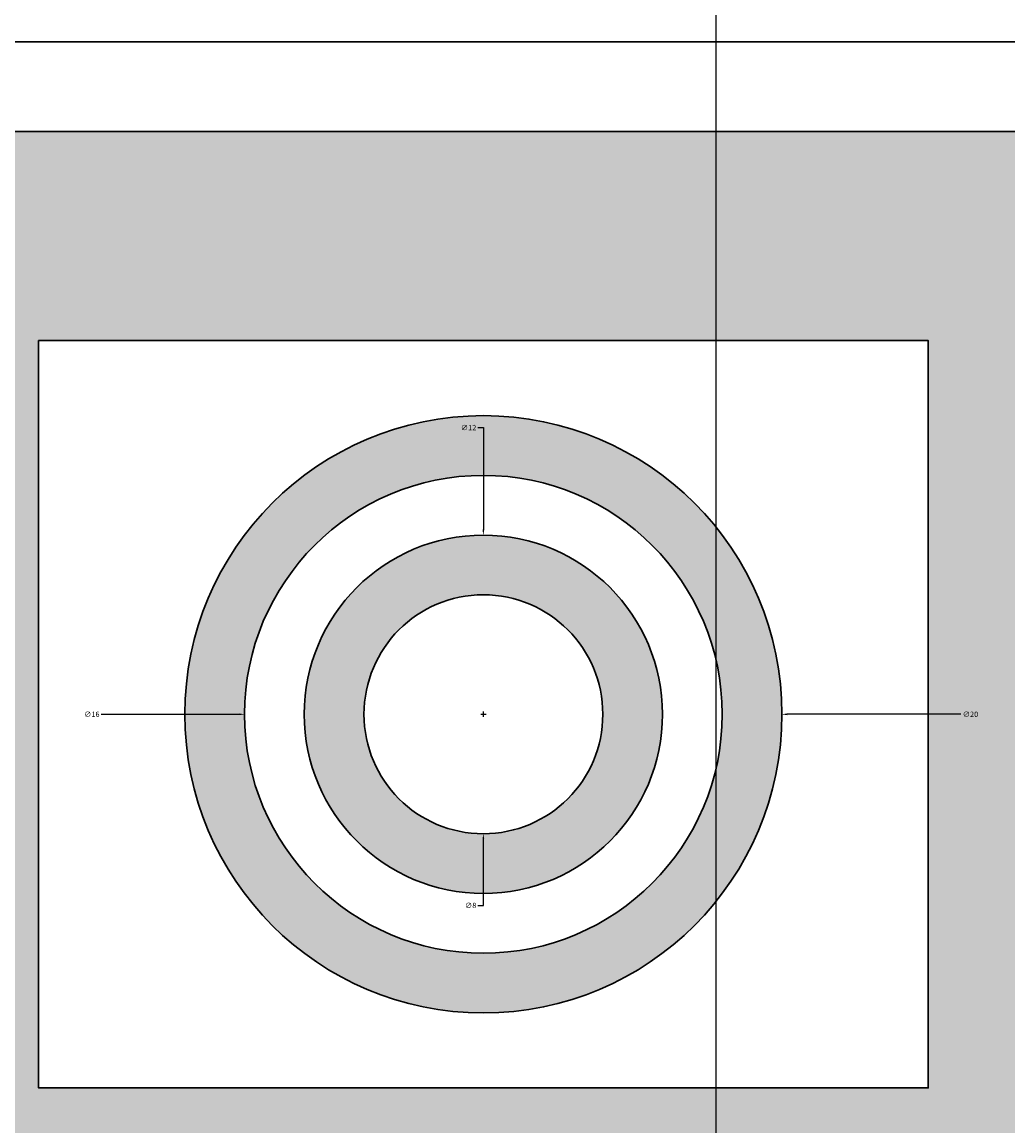
# Model space of a CAD drawing. Units: millimetres. Extents: x -8 to 285, y 5 to 221.
# Tile 20 of 30: x 208 to 241, y 66 to 103. Entities that reach past the tile are written whole.
import ezdxf

# ---------------------------------------------------------------- set-up
doc = ezdxf.new("R2010")
doc.units = ezdxf.units.MM
for name, color, linetype, lineweight in [('A-ANNO-DIMS', 2, 'Continuous', 18), ('E-EQPM-PATT', 252, 'Continuous', 13), ('E-POWR-INVR', 7, 'Continuous', 30)]:
    doc.layers.add(name, color=color, linetype=linetype, lineweight=lineweight)
doc.styles.get("Standard").update_dxf_attribs({"font": 'arial.ttf'})
doc.dimstyles.get("Standard").update_dxf_attribs({"dimtxt": 0.18, "dimasz": 0.18, "dimexe": 0.18, "dimexo": 0.0625, "dimgap": 0.09, "dimtad": 0, "dimtih": 1, "dimtoh": 1, "dimdec": 4, "dimzin": 0, "dimdsep": 46, "dimtxsty": 'Standard', "dimcen": 0.09, "dimadec": 0, "dimazin": 0, "dimtfac": 1, "dimtdec": 4, "dimtofl": 0, "dimtmove": 0, "dimatfit": 3, "dimfxl": 1, "dimtolj": 1, "dimtzin": 0, "dimarcsym": 0})

# ---------------------------------------------------------------- blocks, each defined once
blk = doc.blocks.new('*D14')
at = {"layer": 'A-ANNO-DIMS', "color": 0, "lineweight": -2, "transparency": 16777216}
for p, q in [((189.039, 137.013), (189.039, 5.222)), ((230.967, 137.013), (230.967, 5.222)), ((189.219, 5.402), (209.606, 5.402)), ((230.787, 5.402), (210.4, 5.402))]:
    blk.add_line(p, q, dxfattribs=at)
at = {"layer": 'A-ANNO-DIMS', "color": 0, "transparency": 16777216}
for points in [[(189.219, 5.432), (189.219, 5.372), (189.039, 5.402)], [(230.787, 5.432), (230.787, 5.372), (230.967, 5.402)]]:
    blk.add_solid(points, dxfattribs=at)
at = {"layer": 'Defpoints', "color": 0, "transparency": 16777216}
for p in [(189.039, 137.075), (230.967, 137.075), (230.967, 5.402)]:
    blk.add_point(p, dxfattribs=at)
at = {"layer": 'A-ANNO-DIMS', "color": 0, "transparency": 16777216, "insert": (210.003, 5.402), "char_height": 0.18, "attachment_point": 5}
blk.add_mtext('\\A1;41.93', dxfattribs=at)
blk = doc.blocks.new('*D31')
at = {"layer": 'A-ANNO-DIMS', "color": 0, "lineweight": -2, "transparency": 16777216}
for p, q in [((223.18, 80.093), (223.18, 80.273)), ((223.09, 80.183), (223.27, 80.183)), ((239.18, 80.183), (233.36, 80.183))]:
    blk.add_line(p, q, dxfattribs=at)
at = {"layer": 'A-ANNO-DIMS', "color": 0, "transparency": 16777216}
blk.add_solid([(233.36, 80.213), (233.36, 80.153), (233.18, 80.183)], dxfattribs=at)
at = {"layer": 'Defpoints', "color": 0, "transparency": 16777216}
for p in [(213.18, 80.183), (233.18, 80.183)]:
    blk.add_point(p, dxfattribs=at)
at = {"layer": 'A-ANNO-DIMS', "color": 0, "transparency": 16777216, "insert": (239.497, 80.183), "char_height": 0.18, "attachment_point": 5}
blk.add_mtext('\\A1;∅20', dxfattribs=at)
blk = doc.blocks.new('*D32')
at = {"layer": 'A-ANNO-DIMS', "color": 0, "lineweight": -2, "transparency": 16777216}
for p, q in [((223.18, 80.093), (223.18, 80.273)), ((210.38, 80.183), (215, 80.183)), ((223.09, 80.183), (223.27, 80.183))]:
    blk.add_line(p, q, dxfattribs=at)
at = {"layer": 'A-ANNO-DIMS', "color": 0, "transparency": 16777216}
blk.add_solid([(215, 80.213), (215, 80.153), (215.18, 80.183)], dxfattribs=at)
at = {"layer": 'Defpoints', "color": 0, "transparency": 16777216}
for p in [(215.18, 80.183), (231.18, 80.183)]:
    blk.add_point(p, dxfattribs=at)
at = {"layer": 'A-ANNO-DIMS', "color": 0, "transparency": 16777216, "insert": (210.063, 80.183), "char_height": 0.18, "attachment_point": 5}
blk.add_mtext('\\A1;∅16', dxfattribs=at)
blk = doc.blocks.new('*D33')
at = {"layer": 'A-ANNO-DIMS', "color": 0, "lineweight": -2, "transparency": 16777216}
for p, q in [((223, 89.783), (223.18, 89.783)), ((223.18, 89.783), (223.18, 86.363)), ((223.18, 80.093), (223.18, 80.273)), ((223.09, 80.183), (223.27, 80.183))]:
    blk.add_line(p, q, dxfattribs=at)
at = {"layer": 'A-ANNO-DIMS', "color": 0, "transparency": 16777216}
blk.add_solid([(223.21, 86.363), (223.15, 86.363), (223.18, 86.183)], dxfattribs=at)
at = {"layer": 'Defpoints', "color": 0, "transparency": 16777216}
for p in [(223.18, 86.183), (223.18, 74.183)]:
    blk.add_point(p, dxfattribs=at)
at = {"layer": 'A-ANNO-DIMS', "color": 0, "transparency": 16777216, "insert": (222.684, 89.783), "char_height": 0.18, "attachment_point": 5}
blk.add_mtext('\\A1;∅12', dxfattribs=at)
blk = doc.blocks.new('*D34')
at = {"layer": 'A-ANNO-DIMS', "color": 0, "lineweight": -2, "transparency": 16777216}
for p, q in [((223.18, 80.093), (223.18, 80.273)), ((223.09, 80.183), (223.27, 80.183)), ((223.18, 73.783), (223.18, 76.003)), ((223, 73.783), (223.18, 73.783))]:
    blk.add_line(p, q, dxfattribs=at)
at = {"layer": 'A-ANNO-DIMS', "color": 0, "transparency": 16777216}
blk.add_solid([(223.15, 76.003), (223.21, 76.003), (223.18, 76.183)], dxfattribs=at)
at = {"layer": 'Defpoints', "color": 0, "transparency": 16777216}
for p in [(223.18, 84.183), (223.18, 76.183)]:
    blk.add_point(p, dxfattribs=at)
at = {"layer": 'A-ANNO-DIMS', "color": 0, "transparency": 16777216, "insert": (222.753, 73.783), "char_height": 0.18, "attachment_point": 5}
blk.add_mtext('\\A1;∅8', dxfattribs=at)

msp = doc.modelspace()

# ---------------------------------------------------------------- hatches: boundary and pattern name
at = {"layer": 'E-EQPM-PATT'}
h = msp.add_hatch(color=256, dxfattribs=at)
h.set_gradient(color1=(175, 217, 170), color2=(175, 217, 170), tint=1)
h.paths.add_polyline_path([(255.6152, 99.7021), (190.9955, 99.7021), (190.9955, 53.4644), (215.8749, 53.4644), (215.8749, 47.6512), (217.2608, 47.6512), (219.2608, 45.6512), (219.2608, 32.6512), (199.2608, 32.6512), (199.2608, 44.4759), (190.9955, 44.4759), (190.9955, 28.2311), (237.8513, 28.2311), (237.8513, 32.6512), (231.5468, 32.6512, -0.5773503), (229.8147, 35.6512), (231.5468, 38.6512), (231.5468, 58.5666), (255.6152, 58.5666)])
h.paths.add_polyline_path([(208.2775, 92.6953), (238.0827, 92.6953), (238.0827, 67.6708), (208.2775, 67.6708)], flags=16)
h.paths.add_polyline_path([(213.1801, 80.183, -1), (233.1801, 80.183, -1)], flags=0)
h.paths.add_polyline_path([(215.1801, 80.183, -1), (231.1801, 80.183, -1)], flags=0)
h.paths.add_polyline_path([(217.1801, 80.183, -1), (229.1801, 80.183, -1)], flags=0)
h.paths.add_polyline_path([(219.1801, 80.183, -1), (227.1801, 80.183, -1)], flags=0)
h.paths.add_polyline_path([(255.6152, 58.5666), (231.5468, 58.5666), (231.5468, 38.6512), (236.3506, 46.9717, -0.5773503), (239.8147, 46.9717), (244.6186, 38.6512), (244.6186, 49.925), (255.6152, 49.925)], flags=17)
h.paths.add_polyline_path([(215.8749, 53.4644), (190.9955, 53.4644), (190.9955, 48.962), (202.4345, 48.962), (202.4345, 47.6512), (215.8749, 47.6512)], flags=17)
h.paths.add_polyline_path([(255.6152, 49.925), (244.6186, 49.925), (244.6186, 38.6512), (246.3506, 35.6512, -0.5773503), (244.6186, 32.6512), (237.8513, 32.6512), (237.8513, 28.2311), (190.9955, 28.2311), (190.9955, 25.6297), (255.6152, 25.6297)])
h.paths.add_polyline_path([(199.2608, 45.6512), (201.2608, 47.6512), (202.4345, 47.6512), (202.4345, 48.962), (190.9955, 48.962), (190.9955, 44.4759), (199.2608, 44.4759)], flags=17)

# ---------------------------------------------------------------- linework, layer by layer
at = {"layer": 'E-POWR-INVR'}
for points in [[(187.9955, 102.7021), (258.6152, 102.7021), (258.6152, 22.6297), (187.9955, 22.6297)], [(190.9955, 99.7021), (255.6152, 99.7021), (255.6152, 25.6297), (190.9955, 25.6297)], [(208.2775, 92.6953), (238.0827, 92.6953), (238.0827, 67.6708), (208.2775, 67.6708)]]:
    msp.add_lwpolyline(points, close=True, dxfattribs=at)
for radius in [10, 8, 6, 4]:
    msp.add_circle((223.1801, 80.183), radius, dxfattribs=at)

# ---------------------------------------------------------------- dimensions: what is measured, and where the dimension line sits
at = {"layer": 'A-ANNO-DIMS'}
dim = msp.add_linear_dim(base=(230.9672, 5.402), p1=(189.039, 137.0752), p2=(230.9672, 137.0752), dimstyle='Standard', override={"dimdec": 2, "dimlfac": 1, "dimrnd": 0, "dimzin": 0, "dimdsep": 46, "dimlunit": 2}, dxfattribs=at)
dim.commit()
dim.dimension.update_dxf_attribs({"geometry": '*D14', "text_midpoint": (210.0031, 5.402)})
for p1, p2, picture, middle in [((223.1802, 74.183), (223.18, 86.183), '*D33', (222.684, 89.783)), ((223.1802, 84.183), (223.18, 76.183), '*D34', (222.7528, 73.783)), ((231.1801, 80.183), (215.1801, 80.183), '*D32', (210.3801, 80.183)), ((213.1801, 80.183), (233.1801, 80.183), '*D31', (239.1801, 80.183))]:
    dim = msp.add_diameter_dim_2p(p1=p1, p2=p2, dimstyle='Standard', override={"dimdec": 0, "dimlfac": 1, "dimrnd": 0, "dimzin": 0, "dimdsep": 46, "dimlunit": 2}, dxfattribs=at)
    dim.commit()
    dim.dimension.update_dxf_attribs({"geometry": picture, "text_midpoint": middle, "dimtype": 163})

doc.saveas('drawing.dxf')
